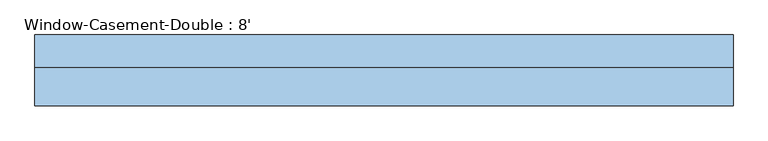
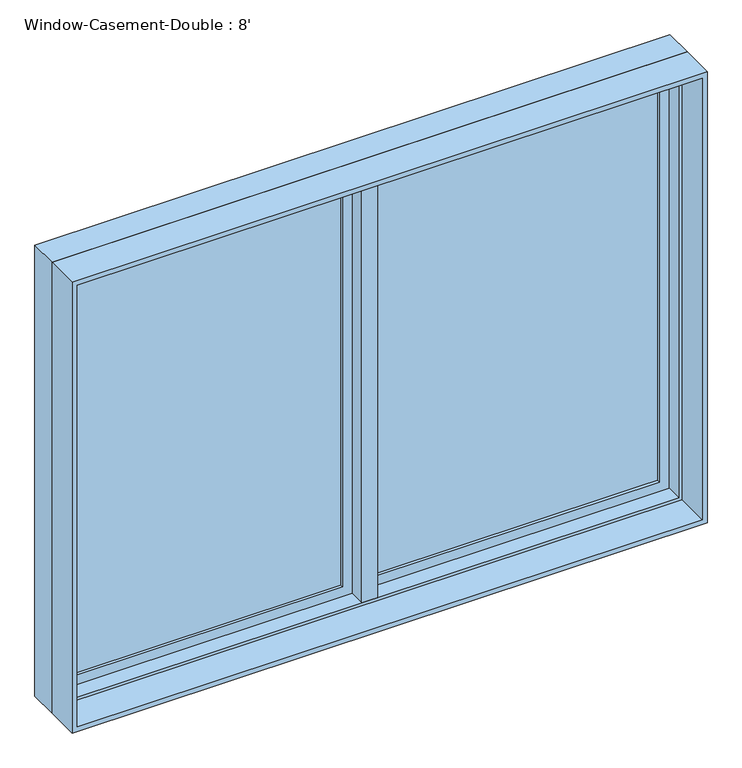
"""IFC4 building model written with IfcOpenShell, lengths in millimetres: window geometry, Window-Casement-Double : 8'."""

from ifc_helpers import new_model, si_unit, frame, origin, place, context, project, spatial, polyline, outline, extrude, faceted_brep, source, transform, mapped, element, save


def window_casement_double_8_9ae172a2(model_context):
    return source(origin(), model_context, "Body", "SolidModel", [
        faceted_brep([(9.525, 133.35, 2730.5), (-9.525, 133.35, 2730.5), (-9.525, 82.55, 2730.5), (9.525, 82.55, 2730.5), (9.525, 133.35, 927.1), (9.525, 82.55, 927.1), (-9.525, 82.55, 927.1), (-9.525, 133.35, 927.1), (-9.525, 82.55, 946.15), (-9.525, 82.55, 2711.45), (-30.1625, 82.55, 946.15), (-30.1625, 82.55, 2711.45), (-30.1625, 19.05, 946.15), (-30.1625, 19.05, 2711.45), (30.1625, 19.05, 946.15), (30.1625, 19.05, 2711.45), (30.1625, 82.55, 946.15), (30.1625, 82.55, 2711.45), (9.525, 82.55, 946.15), (9.525, 82.55, 2711.45)], [[[0, 1, 2, 3]], [[4, 5, 6, 7]], [[1, 0, 4, 7]], [[2, 1, 7, 6, 8, 9]], [[9, 8, 10, 11]], [[11, 10, 12, 13]], [[13, 12, 14, 15]], [[15, 14, 16, 17]], [[17, 16, 18, 19]], [[0, 3, 19, 18, 5, 4]], [[18, 8, 6, 5]], [[9, 19, 3, 2]], [[8, 18, 16, 14, 12, 10]], [[19, 9, 11, 13, 15, 17]]]),
        extrude(outline(polyline([(-66.675, 114.3), (-66.675, 107.95), (-1149.35, 107.95), (-1149.35, 114.3), (-66.675, 114.3)])), frame((0.0, 0.0, 984.25), z_axis=(0.0, 0.0, 1.0), x_axis=(1.0, 0.0, 0.0)), (0.0, 0.0, 1.0), 1689.1),
        extrude(outline(polyline([(-1149.35, 95.25), (-1149.35, 101.6), (-66.675, 101.6), (-66.675, 95.25), (-1149.35, 95.25)])), frame((0.0, 0.0, 984.25), z_axis=(0.0, 0.0, 1.0), x_axis=(1.0, 0.0, 0.0)), (0.0, 0.0, 1.0), 1689.1),
        extrude(outline(polyline([(1149.35, 114.3), (1149.35, 107.95), (66.675, 107.95), (66.675, 114.3), (1149.35, 114.3)])), frame((0.0, 0.0, 984.25), z_axis=(0.0, 0.0, 1.0), x_axis=(1.0, 0.0, 0.0)), (0.0, 0.0, 1.0), 1689.1),
        extrude(outline(polyline([(66.675, 95.25), (66.675, 101.6), (1149.35, 101.6), (1149.35, 95.25), (66.675, 95.25)])), frame((0.0, 0.0, 984.25), z_axis=(0.0, 0.0, 1.0), x_axis=(1.0, 0.0, 0.0)), (0.0, 0.0, 1.0), 1689.1),
        extrude(outline(polyline([(2730.5, -1206.5), (927.1, -1206.5), (927.1, -9.525), (2730.5, -9.525), (2730.5, -1206.5)]), holes=[polyline([(2673.35, -66.675), (984.25, -66.675), (984.25, -1149.35), (2673.35, -1149.35), (2673.35, -66.675)])]), frame((0.0, 82.55, 0.0), z_axis=(0.0, 1.0, 0.0), x_axis=(0.0, 0.0, 1.0)), (0.0, 0.0, 1.0), 44.45),
        extrude(outline(polyline([(927.1, 1206.5), (2730.5, 1206.5), (2730.5, 9.525), (927.1, 9.525), (927.1, 1206.5)]), holes=[polyline([(984.25, 66.675), (2673.35, 66.675), (2673.35, 1149.35), (984.25, 1149.35), (984.25, 66.675)])]), frame((0.0, 82.55, 0.0), z_axis=(0.0, 1.0, 0.0), x_axis=(0.0, 0.0, 1.0)), (0.0, 0.0, 1.0), 44.45),
        extrude(outline(polyline([(2743.2, -1219.2), (914.4, -1219.2), (914.4, 1219.2), (2743.2, 1219.2), (2743.2, -1219.2)]), holes=[polyline([(2724.15, 1200.15), (933.45, 1200.15), (933.45, -1200.15), (2724.15, -1200.15), (2724.15, 1200.15)])]), frame((0.0, -114.3, 0.0), z_axis=(0.0, 1.0, 0.0), x_axis=(0.0, 0.0, 1.0)), (0.0, 0.0, 1.0), 133.35),
        faceted_brep([(1187.45, 82.55, 2711.45), (1187.45, 19.05, 2711.45), (-1187.45, 19.05, 2711.45), (-1187.45, 82.55, 2711.45), (1206.5, 133.35, 2730.5), (1206.5, 82.55, 2730.5), (-1206.5, 82.55, 2730.5), (-1206.5, 133.35, 2730.5), (1219.2, 19.05, 2743.2), (1219.2, 133.35, 2743.2), (-1219.2, 133.35, 2743.2), (-1219.2, 19.05, 2743.2), (-1187.45, 19.05, 946.15), (-1187.45, 82.55, 946.15), (-1206.5, 82.55, 927.1), (-1206.5, 133.35, 927.1), (-1219.2, 133.35, 914.4), (-1219.2, 19.05, 914.4), (1187.45, 19.05, 946.15), (1187.45, 82.55, 946.15), (1206.5, 82.55, 927.1), (1206.5, 133.35, 927.1), (1219.2, 133.35, 914.4), (1219.2, 19.05, 914.4)], [[[0, 1, 2, 3]], [[4, 5, 6, 7]], [[8, 9, 10, 11]], [[3, 2, 12, 13]], [[7, 6, 14, 15]], [[11, 10, 16, 17]], [[13, 12, 18, 19]], [[15, 14, 20, 21]], [[17, 16, 22, 23]], [[11, 17, 23, 8], [1, 18, 12, 2]], [[19, 18, 1, 0]], [[5, 20, 14, 6], [3, 13, 19, 0]], [[21, 20, 5, 4]], [[23, 22, 9, 8]], [[9, 22, 16, 10], [7, 15, 21, 4]]]),
    ])


if __name__ == "__main__":
    model = new_model("IFC4")
    model_context = context("Model", 3, world=origin())
    ifc_project = project(units=[si_unit("LENGTHUNIT", "METRE", prefix="MILLI")], contexts=[model_context])
    site = spatial("IfcSite", under=ifc_project)
    building = spatial("IfcBuilding", under=site)
    placement = place(None, origin())
    window_casement_double_8_shape = window_casement_double_8_9ae172a2(model_context)
    element("IfcWindow", 1, ObjectType="Window-Casement-Double : 8'", at=placement, inside=building, context=model_context, shape_type="MappedRepresentation", body=[
        mapped(window_casement_double_8_shape, transform((0.0, 0.0, 0.0), x_axis=(1.0, 0.0, 0.0), y_axis=(0.0, 1.0, 0.0), z_axis=(0.0, 0.0, 1.0))),
    ])
    save(model, "model.ifc")

# Revit data of these elements
# Type "Window-Casement-Double : 8'"
#   Type Mark = "27"
#   Fire Rating = "0.5h"
#   Assembly Code = "B2020100"
#   Analytic Construction = "Double glazing - domestic"
#   Frame Extension [instance default] = 0' - 0 1/4"
#   Window Inset [instance default] = 0' - 0"
#   Wall Thickness [instance default] = 0' - 6"
#   Interior Wall Closure [instance default] = 0' - 2 1/4"
#   Half Width = 4' - 0"
#   Visual Light Transmittance = 0.81
#   Thermal Resistance (R) = 1.8146 (h·ft²·°F)/BTU
#   Solar Heat Gain Coefficient = 0.76
#   Rough Width = 8' - 0 1/2"
#   Rough Height = 6' - 0 1/2"
#   Height = 6' - 0"
#   Heat Transfer Coefficient (U) = 0.5511 BTU/(h·ft²·°F)
#   Exterior Wall Closure [instance default] = 0' - 1 1/4"
#   Extension Jamb [instance default] = 0' - 2 1/4"
#   Default Sill Height = 3' - 0"
#   Width = 8' - 0"
#   Muntin Visibility = yes
#   Interior Trim Visibility [instance default] = yes
#   Exterior Trim Visibility [instance default] = yes
#   Extension Jamb Visibility [instance default] = yes
#   Interior Trim Material = Wood - Stained
#   Muntin Pattern = Muntin Pattern_2x2 : Muntin Pattern_2x2
#   Interior Trim = Trim-Window-Interior-Flat : Picture Frame
#   Interior Frame Material = Wood - Stained
#   Glass Panel Material = Glass
#   Exterior Trim Material = Clad - White
#   Exterior Trim = Trim-Window-Exterior-Flat : with Sill
#   Exterior Frame Material = Clad - White
#   Wall Closure = (empty or 0)
# Element 1 (IfcWindow, "Window-Casement-Double : 8'")
#   Wall Thickness = 0' - 9"
#   Extension Jamb = 0' - 5 1/4"
#   Materials on its faces: "Wood - Stained", "Glass", "Clad - White"
# Materials
#   "Wood - Stained": class "Wood", colour RGB 224 178 126, transparency 0, Cost = 0
#   "Glass": class "Glass", colour RGB 0 128 192, transparency 0.75, Description = "Soda Lime Glass", Cost = 0
#   "Clad - White": class "Wood", colour RGB 242 242 238, transparency 0, Cost = 0
